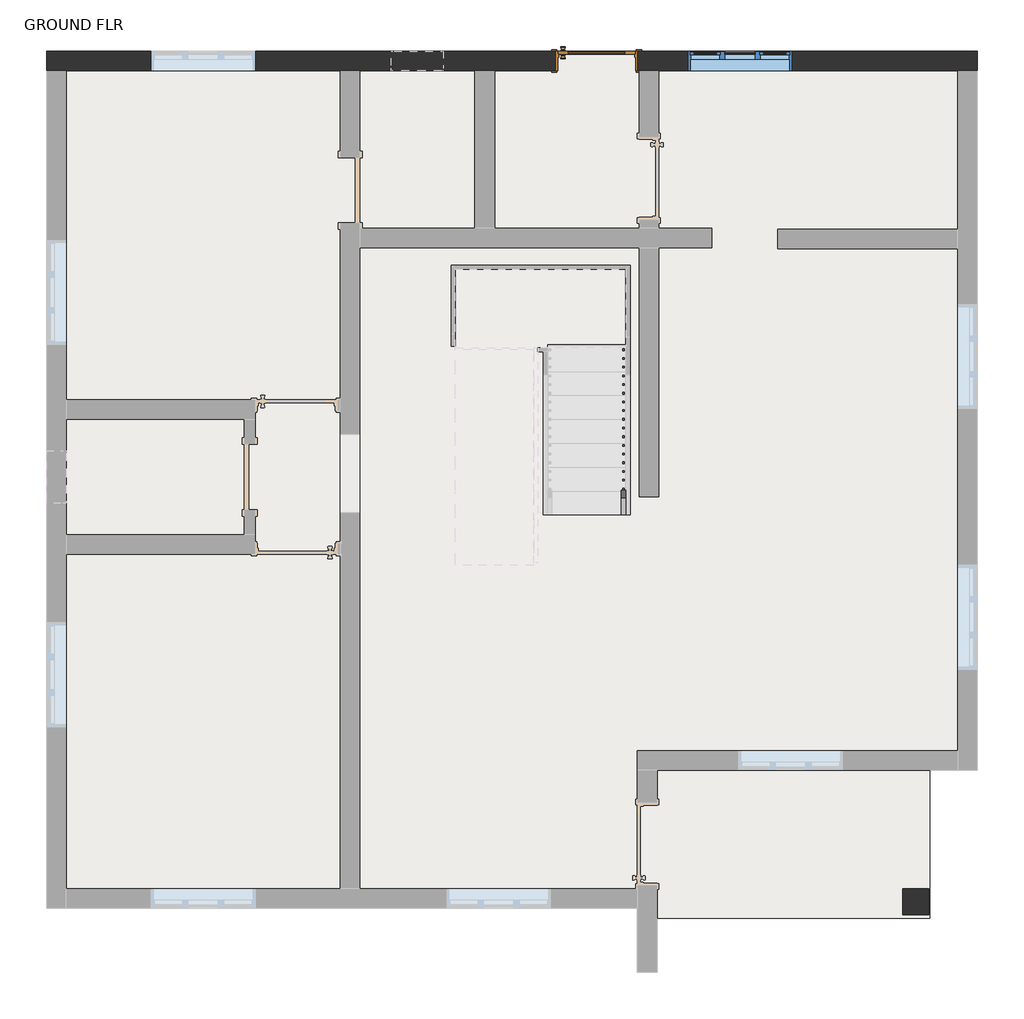
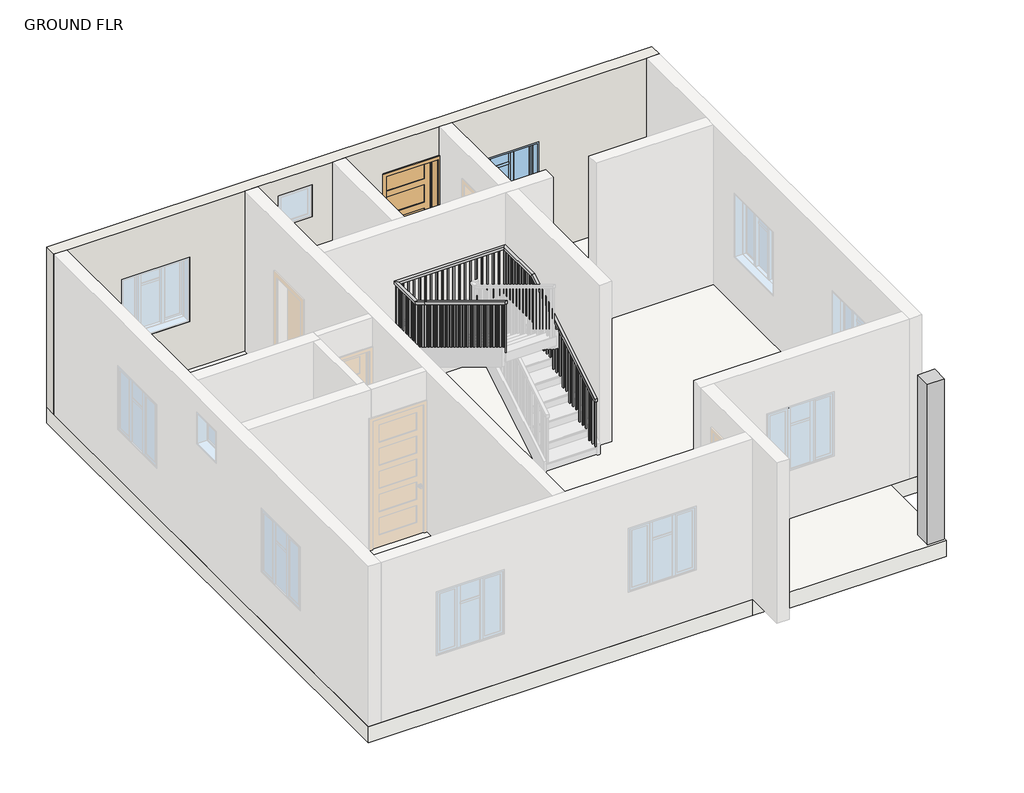
# One storey, part 2 of 3: 1 column, 1 door, 1 railing, 1 slab, 1 wall, 1 window.
"""IFC4 building model written with IfcOpenShell, lengths in millimetres."""

from ifc_helpers import new_model, si_unit, frame, origin, place, context, project, spatial, polyline, outline, extrude, faceted_brep, transform, mapped, element, save
from components import rectangular_column_1_x_1_0efb18cf, door_d793c26e, window_casement_triple_middle_transom_window_4_x_4_1416bf83

model = new_model("IFC4")

# Units and contexts
model_context = context("Model", 3, world=origin())
ifc_project = project(units=[si_unit("LENGTHUNIT", "METRE", prefix="MILLI")], contexts=[model_context])

# Site, building, storey
site = spatial("IfcSite", under=ifc_project)
building = spatial("IfcBuilding", under=site)
storey = spatial("IfcBuildingStorey", under=building, Name="GROUND FLR", Elevation=609.6)

# Column
placement = place(None, origin())
rectangular_column_1_x_1_shape = rectangular_column_1_x_1_0efb18cf(model_context)
element("IfcColumn", 1, ObjectType="Rectangular Column : 1' x 1'", at=placement, inside=storey, context=model_context, shape_type="MappedRepresentation", body=[
    mapped(rectangular_column_1_x_1_shape, transform((-1992.6206632, -7773.7948807, 0.0), x_axis=(1.0, 0.0, 0.0), y_axis=(0.0, 1.0, 0.0), z_axis=(0.0, 0.0, 1.0))),
])

# Door
door_shape = door_d793c26e(model_context)
element("IfcDoor", 2, ObjectType="Door-Interior-Single-5_Panel_Vert-Wood : 36\" x 96\"", at=placement, inside=storey, context=model_context, shape_type="MappedRepresentation", body=[
    mapped(door_shape, transform((-5721.0431792, 2059.1801193, 609.6), x_axis=(1.0, 0.0, 0.0), y_axis=(0.0, 1.0, 0.0), z_axis=(0.0, 0.0, 1.0))),
])

# Railing
element("IfcRailing", 3, ObjectType="Handrail - Rectangular", at=placement, inside=storey, context=model_context, shape_type="SolidModel", body=[
    faceted_brep([(-5431.2481169, -3250.5249317, 1693.3333333), (-5431.2481169, -3250.5249317, 1633.9318731), (-5380.4481169, -3250.5249317, 1633.9318731), (-5380.4481169, -3250.5249317, 1693.3333333), (-5431.2481169, -1294.7249317, 2878.6666667), (-5431.2481169, -1280.5325223, 2827.8666667), (-5380.4481169, -1280.5325223, 2827.8666667), (-5380.4481169, -1294.7249317, 2878.6666667), (-5431.2481169, -431.1249317, 2878.6666667), (-5431.2481169, -431.1249317, 2827.8666667), (-5380.4481169, -380.3249317, 2827.8666667), (-5380.4481169, -380.3249317, 2878.6666667), (-7321.2431792, -431.1249317, 2878.6666667), (-7321.2431792, -431.1249317, 2827.8666667), (-7372.0431792, -380.3249317, 2827.8666667), (-7372.0431792, -380.3249317, 2878.6666667), (-7321.2431792, -1015.3249317, 2878.6666667), (-7321.2431792, -1029.5173411, 2827.8666667), (-7372.0431792, -1029.5173411, 2827.8666667), (-7372.0431792, -1015.3249317, 2878.6666667), (-7321.2431792, -1294.7249317, 3048.0), (-7321.2431792, -1321.0546589, 3004.5559502), (-7372.0431792, -1321.0546589, 3004.5559502), (-7372.0431792, -1294.7249317, 3048.0), (-7321.2431792, -3809.3249317, 4572.0), (-7372.0431792, -3809.3249317, 4572.0), (-7372.0431792, -3809.3249317, 4512.5985397), (-7321.2431792, -3809.3249317, 4512.5985397)], [[[0, 1, 2, 3]], [[1, 0, 4, 5]], [[2, 1, 5, 6]], [[3, 2, 6, 7]], [[0, 3, 7, 4]], [[5, 4, 8, 9]], [[6, 5, 9, 10]], [[7, 6, 10, 11]], [[4, 7, 11, 8]], [[9, 8, 12, 13]], [[10, 9, 13, 14]], [[11, 10, 14, 15]], [[8, 11, 15, 12]], [[13, 12, 16, 17]], [[14, 13, 17, 18]], [[15, 14, 18, 19]], [[12, 15, 19, 16]], [[17, 16, 20, 21]], [[18, 17, 21, 22]], [[19, 18, 22, 23]], [[16, 19, 23, 20]], [[24, 25, 26, 27]], [[21, 20, 24, 27]], [[22, 21, 27, 26]], [[23, 22, 26, 25]], [[20, 23, 25, 24]]]),
    extrude(outline(polyline([(-3742.6499317, 4472.1894488), (-3723.5999317, 4460.6439943), (-3723.5999317, 3488.2666667), (-3742.6499317, 3488.2666667), (-3742.6499317, 4472.1894488)])), frame((-7356.1681792, 0.0, 0.0), z_axis=(1.0, 0.0, 0.0), x_axis=(0.0, 1.0, 0.0)), (0.0, 0.0, 1.0), 19.05),
    extrude(outline(polyline([(-3641.0499317, 4410.6136913), (-3621.9999317, 4399.0682367), (-3621.9999317, 3488.2666667), (-3641.0499317, 3488.2666667), (-3641.0499317, 4410.6136913)])), frame((-7356.1681792, 0.0, 0.0), z_axis=(1.0, 0.0, 0.0), x_axis=(0.0, 1.0, 0.0)), (0.0, 0.0, 1.0), 19.05),
    extrude(outline(polyline([(-3539.4499317, 4349.0379337), (-3520.3999317, 4337.4924791), (-3520.3999317, 3488.2666667), (-3539.4499317, 3488.2666667), (-3539.4499317, 4349.0379337)])), frame((-7356.1681792, 0.0, 0.0), z_axis=(1.0, 0.0, 0.0), x_axis=(0.0, 1.0, 0.0)), (0.0, 0.0, 1.0), 19.05),
    extrude(outline(polyline([(-3437.8499317, 4287.4621761), (-3418.7999317, 4275.9167216), (-3418.7999317, 3318.9333333), (-3437.8499317, 3318.9333333), (-3437.8499317, 4287.4621761)])), frame((-7356.1681792, 0.0, 0.0), z_axis=(1.0, 0.0, 0.0), x_axis=(0.0, 1.0, 0.0)), (0.0, 0.0, 1.0), 19.05),
    extrude(outline(polyline([(-3336.2499317, 4225.8864185), (-3317.1999317, 4214.340964), (-3317.1999317, 3318.9333333), (-3336.2499317, 3318.9333333), (-3336.2499317, 4225.8864185)])), frame((-7356.1681792, 0.0, 0.0), z_axis=(1.0, 0.0, 0.0), x_axis=(0.0, 1.0, 0.0)), (0.0, 0.0, 1.0), 19.05),
    extrude(outline(polyline([(-3234.6499317, 4164.310661), (-3215.5999317, 4152.7652064), (-3215.5999317, 3149.6), (-3234.6499317, 3149.6), (-3234.6499317, 4164.310661)])), frame((-7356.1681792, 0.0, 0.0), z_axis=(1.0, 0.0, 0.0), x_axis=(0.0, 1.0, 0.0)), (0.0, 0.0, 1.0), 19.05),
    extrude(outline(polyline([(-3133.0499317, 4102.7349034), (-3113.9999317, 4091.1894488), (-3113.9999317, 3149.6), (-3133.0499317, 3149.6), (-3133.0499317, 4102.7349034)])), frame((-7356.1681792, 0.0, 0.0), z_axis=(1.0, 0.0, 0.0), x_axis=(0.0, 1.0, 0.0)), (0.0, 0.0, 1.0), 19.05),
    extrude(outline(polyline([(-3031.4499317, 4041.1591458), (-3012.3999317, 4029.6136913), (-3012.3999317, 3149.6), (-3031.4499317, 3149.6), (-3031.4499317, 4041.1591458)])), frame((-7356.1681792, 0.0, 0.0), z_axis=(1.0, 0.0, 0.0), x_axis=(0.0, 1.0, 0.0)), (0.0, 0.0, 1.0), 19.05),
    extrude(outline(polyline([(-2929.8499317, 3979.5833882), (-2910.7999317, 3968.0379337), (-2910.7999317, 2980.2666667), (-2929.8499317, 2980.2666667), (-2929.8499317, 3979.5833882)])), frame((-7356.1681792, 0.0, 0.0), z_axis=(1.0, 0.0, 0.0), x_axis=(0.0, 1.0, 0.0)), (0.0, 0.0, 1.0), 19.05),
    extrude(outline(polyline([(-2828.2499317, 3918.0076307), (-2809.1999317, 3906.4621761), (-2809.1999317, 2980.2666667), (-2828.2499317, 2980.2666667), (-2828.2499317, 3918.0076307)])), frame((-7356.1681792, 0.0, 0.0), z_axis=(1.0, 0.0, 0.0), x_axis=(0.0, 1.0, 0.0)), (0.0, 0.0, 1.0), 19.05),
    extrude(outline(polyline([(-2726.6499317, 3856.4318731), (-2707.5999317, 3844.8864185), (-2707.5999317, 2980.2666667), (-2726.6499317, 2980.2666667), (-2726.6499317, 3856.4318731)])), frame((-7356.1681792, 0.0, 0.0), z_axis=(1.0, 0.0, 0.0), x_axis=(0.0, 1.0, 0.0)), (0.0, 0.0, 1.0), 19.05),
    extrude(outline(polyline([(-2625.0499317, 3794.8561155), (-2605.9999317, 3783.310661), (-2605.9999317, 2810.9333333), (-2625.0499317, 2810.9333333), (-2625.0499317, 3794.8561155)])), frame((-7356.1681792, 0.0, 0.0), z_axis=(1.0, 0.0, 0.0), x_axis=(0.0, 1.0, 0.0)), (0.0, 0.0, 1.0), 19.05),
    extrude(outline(polyline([(-2523.4499317, 3733.2803579), (-2504.3999317, 3721.7349034), (-2504.3999317, 2810.9333333), (-2523.4499317, 2810.9333333), (-2523.4499317, 3733.2803579)])), frame((-7356.1681792, 0.0, 0.0), z_axis=(1.0, 0.0, 0.0), x_axis=(0.0, 1.0, 0.0)), (0.0, 0.0, 1.0), 19.05),
    extrude(outline(polyline([(-2421.8499317, 3671.7046004), (-2402.7999317, 3660.1591458), (-2402.7999317, 2810.9333333), (-2421.8499317, 2810.9333333), (-2421.8499317, 3671.7046004)])), frame((-7356.1681792, 0.0, 0.0), z_axis=(1.0, 0.0, 0.0), x_axis=(0.0, 1.0, 0.0)), (0.0, 0.0, 1.0), 19.05),
    extrude(outline(polyline([(-2320.2499317, 3610.1288428), (-2301.1999317, 3598.5833882), (-2301.1999317, 2641.6), (-2320.2499317, 2641.6), (-2320.2499317, 3610.1288428)])), frame((-7356.1681792, 0.0, 0.0), z_axis=(1.0, 0.0, 0.0), x_axis=(0.0, 1.0, 0.0)), (0.0, 0.0, 1.0), 19.05),
    extrude(outline(polyline([(-2218.6499317, 3548.5530852), (-2199.5999317, 3537.0076307), (-2199.5999317, 2641.6), (-2218.6499317, 2641.6), (-2218.6499317, 3548.5530852)])), frame((-7356.1681792, 0.0, 0.0), z_axis=(1.0, 0.0, 0.0), x_axis=(0.0, 1.0, 0.0)), (0.0, 0.0, 1.0), 19.05),
    extrude(outline(polyline([(-2117.0499317, 3486.9773276), (-2097.9999317, 3475.4318731), (-2097.9999317, 2472.2666667), (-2117.0499317, 2472.2666667), (-2117.0499317, 3486.9773276)])), frame((-7356.1681792, 0.0, 0.0), z_axis=(1.0, 0.0, 0.0), x_axis=(0.0, 1.0, 0.0)), (0.0, 0.0, 1.0), 19.05),
    extrude(outline(polyline([(-2015.4499317, 3425.40157), (-1996.3999317, 3413.8561155), (-1996.3999317, 2472.2666667), (-2015.4499317, 2472.2666667), (-2015.4499317, 3425.40157)])), frame((-7356.1681792, 0.0, 0.0), z_axis=(1.0, 0.0, 0.0), x_axis=(0.0, 1.0, 0.0)), (0.0, 0.0, 1.0), 19.05),
    extrude(outline(polyline([(-1913.8499317, 3363.8258125), (-1894.7999317, 3352.2803579), (-1894.7999317, 2472.2666667), (-1913.8499317, 2472.2666667), (-1913.8499317, 3363.8258125)])), frame((-7356.1681792, 0.0, 0.0), z_axis=(1.0, 0.0, 0.0), x_axis=(0.0, 1.0, 0.0)), (0.0, 0.0, 1.0), 19.05),
    extrude(outline(polyline([(-1812.2499317, 3302.2500549), (-1793.1999317, 3290.7046004), (-1793.1999317, 2302.9333333), (-1812.2499317, 2302.9333333), (-1812.2499317, 3302.2500549)])), frame((-7356.1681792, 0.0, 0.0), z_axis=(1.0, 0.0, 0.0), x_axis=(0.0, 1.0, 0.0)), (0.0, 0.0, 1.0), 19.05),
    extrude(outline(polyline([(-1710.6499317, 3240.6742973), (-1691.5999317, 3229.1288428), (-1691.5999317, 2302.9333333), (-1710.6499317, 2302.9333333), (-1710.6499317, 3240.6742973)])), frame((-7356.1681792, 0.0, 0.0), z_axis=(1.0, 0.0, 0.0), x_axis=(0.0, 1.0, 0.0)), (0.0, 0.0, 1.0), 19.05),
    extrude(outline(polyline([(-1609.0499317, 3179.0985397), (-1589.9999317, 3167.5530852), (-1589.9999317, 2302.9333333), (-1609.0499317, 2302.9333333), (-1609.0499317, 3179.0985397)])), frame((-7356.1681792, 0.0, 0.0), z_axis=(1.0, 0.0, 0.0), x_axis=(0.0, 1.0, 0.0)), (0.0, 0.0, 1.0), 19.05),
    extrude(outline(polyline([(-1507.4499317, 3117.5227822), (-1488.3999317, 3105.9773276), (-1488.3999317, 2133.6), (-1507.4499317, 2133.6), (-1507.4499317, 3117.5227822)])), frame((-7356.1681792, 0.0, 0.0), z_axis=(1.0, 0.0, 0.0), x_axis=(0.0, 1.0, 0.0)), (0.0, 0.0, 1.0), 19.05),
    extrude(outline(polyline([(-1405.8499317, 3055.9470246), (-1386.7999317, 3044.40157), (-1386.7999317, 2133.6), (-1405.8499317, 2133.6), (-1405.8499317, 3055.9470246)])), frame((-7356.1681792, 0.0, 0.0), z_axis=(1.0, 0.0, 0.0), x_axis=(0.0, 1.0, 0.0)), (0.0, 0.0, 1.0), 19.05),
    extrude(outline(polyline([(-1228.0499317, 2948.1894488), (-1208.9999317, 2936.6439943), (-1208.9999317, 1964.2666667), (-1228.0499317, 1964.2666667), (-1228.0499317, 2948.1894488)])), frame((-7356.1681792, 0.0, 0.0), z_axis=(1.0, 0.0, 0.0), x_axis=(0.0, 1.0, 0.0)), (0.0, 0.0, 1.0), 19.05),
    extrude(outline(polyline([(-1126.4499317, 2886.6136913), (-1107.3999317, 2875.0682367), (-1107.3999317, 1964.2666667), (-1126.4499317, 1964.2666667), (-1126.4499317, 2886.6136913)])), frame((-7356.1681792, 0.0, 0.0), z_axis=(1.0, 0.0, 0.0), x_axis=(0.0, 1.0, 0.0)), (0.0, 0.0, 1.0), 19.05),
    extrude(outline(polyline([(-7356.1681792, -1005.7999317), (-7337.1181792, -1005.7999317), (-7337.1181792, -1024.8499317), (-7356.1681792, -1024.8499317), (-7356.1681792, -1005.7999317)])), frame((0.0, 0.0, 1964.2666667), z_axis=(0.0, 0.0, 1.0), x_axis=(1.0, 0.0, 0.0)), (0.0, 0.0, 1.0), 863.6),
    extrude(outline(polyline([(-7356.1681792, -904.1999317), (-7337.1181792, -904.1999317), (-7337.1181792, -923.2499317), (-7356.1681792, -923.2499317), (-7356.1681792, -904.1999317)])), frame((0.0, 0.0, 1964.2666667), z_axis=(0.0, 0.0, 1.0), x_axis=(1.0, 0.0, 0.0)), (0.0, 0.0, 1.0), 863.6),
    extrude(outline(polyline([(-7356.1681792, -802.5999317), (-7337.1181792, -802.5999317), (-7337.1181792, -821.6499317), (-7356.1681792, -821.6499317), (-7356.1681792, -802.5999317)])), frame((0.0, 0.0, 1964.2666667), z_axis=(0.0, 0.0, 1.0), x_axis=(1.0, 0.0, 0.0)), (0.0, 0.0, 1.0), 863.6),
    extrude(outline(polyline([(-7356.1681792, -700.9999317), (-7337.1181792, -700.9999317), (-7337.1181792, -720.0499317), (-7356.1681792, -720.0499317), (-7356.1681792, -700.9999317)])), frame((0.0, 0.0, 1964.2666667), z_axis=(0.0, 0.0, 1.0), x_axis=(1.0, 0.0, 0.0)), (0.0, 0.0, 1.0), 863.6),
    extrude(outline(polyline([(-7356.1681792, -599.3999317), (-7337.1181792, -599.3999317), (-7337.1181792, -618.4499317), (-7356.1681792, -618.4499317), (-7356.1681792, -599.3999317)])), frame((0.0, 0.0, 1964.2666667), z_axis=(0.0, 0.0, 1.0), x_axis=(1.0, 0.0, 0.0)), (0.0, 0.0, 1.0), 863.6),
    extrude(outline(polyline([(-7356.1681792, -497.7999317), (-7337.1181792, -497.7999317), (-7337.1181792, -516.8499317), (-7356.1681792, -516.8499317), (-7356.1681792, -497.7999317)])), frame((0.0, 0.0, 1964.2666667), z_axis=(0.0, 0.0, 1.0), x_axis=(1.0, 0.0, 0.0)), (0.0, 0.0, 1.0), 863.6),
    extrude(outline(polyline([(-7326.7231169, -396.1999317), (-7326.7231169, -415.2499317), (-7345.7731169, -415.2499317), (-7345.7731169, -396.1999317), (-7326.7231169, -396.1999317)])), frame((0.0, 0.0, 1964.2666667), z_axis=(0.0, 0.0, 1.0), x_axis=(1.0, 0.0, 0.0)), (0.0, 0.0, 1.0), 863.6),
    extrude(outline(polyline([(-7225.1231169, -396.1999317), (-7225.1231169, -415.2499317), (-7244.1731169, -415.2499317), (-7244.1731169, -396.1999317), (-7225.1231169, -396.1999317)])), frame((0.0, 0.0, 1964.2666667), z_axis=(0.0, 0.0, 1.0), x_axis=(1.0, 0.0, 0.0)), (0.0, 0.0, 1.0), 863.6),
    extrude(outline(polyline([(-7123.5231169, -396.1999317), (-7123.5231169, -415.2499317), (-7142.5731169, -415.2499317), (-7142.5731169, -396.1999317), (-7123.5231169, -396.1999317)])), frame((0.0, 0.0, 1964.2666667), z_axis=(0.0, 0.0, 1.0), x_axis=(1.0, 0.0, 0.0)), (0.0, 0.0, 1.0), 863.6),
    extrude(outline(polyline([(-7021.9231169, -396.1999317), (-7021.9231169, -415.2499317), (-7040.9731169, -415.2499317), (-7040.9731169, -396.1999317), (-7021.9231169, -396.1999317)])), frame((0.0, 0.0, 1964.2666667), z_axis=(0.0, 0.0, 1.0), x_axis=(1.0, 0.0, 0.0)), (0.0, 0.0, 1.0), 863.6),
    extrude(outline(polyline([(-6920.3231169, -396.1999317), (-6920.3231169, -415.2499317), (-6939.3731169, -415.2499317), (-6939.3731169, -396.1999317), (-6920.3231169, -396.1999317)])), frame((0.0, 0.0, 1964.2666667), z_axis=(0.0, 0.0, 1.0), x_axis=(1.0, 0.0, 0.0)), (0.0, 0.0, 1.0), 863.6),
    extrude(outline(polyline([(-6818.7231169, -396.1999317), (-6818.7231169, -415.2499317), (-6837.7731169, -415.2499317), (-6837.7731169, -396.1999317), (-6818.7231169, -396.1999317)])), frame((0.0, 0.0, 1964.2666667), z_axis=(0.0, 0.0, 1.0), x_axis=(1.0, 0.0, 0.0)), (0.0, 0.0, 1.0), 863.6),
    extrude(outline(polyline([(-6717.1231169, -396.1999317), (-6717.1231169, -415.2499317), (-6736.1731169, -415.2499317), (-6736.1731169, -396.1999317), (-6717.1231169, -396.1999317)])), frame((0.0, 0.0, 1964.2666667), z_axis=(0.0, 0.0, 1.0), x_axis=(1.0, 0.0, 0.0)), (0.0, 0.0, 1.0), 863.6),
    extrude(outline(polyline([(-6615.5231169, -396.1999317), (-6615.5231169, -415.2499317), (-6634.5731169, -415.2499317), (-6634.5731169, -396.1999317), (-6615.5231169, -396.1999317)])), frame((0.0, 0.0, 1964.2666667), z_axis=(0.0, 0.0, 1.0), x_axis=(1.0, 0.0, 0.0)), (0.0, 0.0, 1.0), 863.6),
    extrude(outline(polyline([(-6513.9231169, -396.1999317), (-6513.9231169, -415.2499317), (-6532.9731169, -415.2499317), (-6532.9731169, -396.1999317), (-6513.9231169, -396.1999317)])), frame((0.0, 0.0, 1964.2666667), z_axis=(0.0, 0.0, 1.0), x_axis=(1.0, 0.0, 0.0)), (0.0, 0.0, 1.0), 863.6),
    extrude(outline(polyline([(-6412.3231169, -396.1999317), (-6412.3231169, -415.2499317), (-6431.3731169, -415.2499317), (-6431.3731169, -396.1999317), (-6412.3231169, -396.1999317)])), frame((0.0, 0.0, 1964.2666667), z_axis=(0.0, 0.0, 1.0), x_axis=(1.0, 0.0, 0.0)), (0.0, 0.0, 1.0), 863.6),
    extrude(outline(polyline([(-6310.7231169, -396.1999317), (-6310.7231169, -415.2499317), (-6329.7731169, -415.2499317), (-6329.7731169, -396.1999317), (-6310.7231169, -396.1999317)])), frame((0.0, 0.0, 1964.2666667), z_axis=(0.0, 0.0, 1.0), x_axis=(1.0, 0.0, 0.0)), (0.0, 0.0, 1.0), 863.6),
    extrude(outline(polyline([(-6209.1231169, -396.1999317), (-6209.1231169, -415.2499317), (-6228.1731169, -415.2499317), (-6228.1731169, -396.1999317), (-6209.1231169, -396.1999317)])), frame((0.0, 0.0, 1964.2666667), z_axis=(0.0, 0.0, 1.0), x_axis=(1.0, 0.0, 0.0)), (0.0, 0.0, 1.0), 863.6),
    extrude(outline(polyline([(-6107.5231169, -396.1999317), (-6107.5231169, -415.2499317), (-6126.5731169, -415.2499317), (-6126.5731169, -396.1999317), (-6107.5231169, -396.1999317)])), frame((0.0, 0.0, 1964.2666667), z_axis=(0.0, 0.0, 1.0), x_axis=(1.0, 0.0, 0.0)), (0.0, 0.0, 1.0), 863.6),
    extrude(outline(polyline([(-6005.9231169, -396.1999317), (-6005.9231169, -415.2499317), (-6024.9731169, -415.2499317), (-6024.9731169, -396.1999317), (-6005.9231169, -396.1999317)])), frame((0.0, 0.0, 1964.2666667), z_axis=(0.0, 0.0, 1.0), x_axis=(1.0, 0.0, 0.0)), (0.0, 0.0, 1.0), 863.6),
    extrude(outline(polyline([(-5904.3231169, -396.1999317), (-5904.3231169, -415.2499317), (-5923.3731169, -415.2499317), (-5923.3731169, -396.1999317), (-5904.3231169, -396.1999317)])), frame((0.0, 0.0, 1964.2666667), z_axis=(0.0, 0.0, 1.0), x_axis=(1.0, 0.0, 0.0)), (0.0, 0.0, 1.0), 863.6),
    extrude(outline(polyline([(-5802.7231169, -396.1999317), (-5802.7231169, -415.2499317), (-5821.7731169, -415.2499317), (-5821.7731169, -396.1999317), (-5802.7231169, -396.1999317)])), frame((0.0, 0.0, 1964.2666667), z_axis=(0.0, 0.0, 1.0), x_axis=(1.0, 0.0, 0.0)), (0.0, 0.0, 1.0), 863.6),
    extrude(outline(polyline([(-5701.1231169, -396.1999317), (-5701.1231169, -415.2499317), (-5720.1731169, -415.2499317), (-5720.1731169, -396.1999317), (-5701.1231169, -396.1999317)])), frame((0.0, 0.0, 1964.2666667), z_axis=(0.0, 0.0, 1.0), x_axis=(1.0, 0.0, 0.0)), (0.0, 0.0, 1.0), 863.6),
    extrude(outline(polyline([(-5599.5231169, -396.1999317), (-5599.5231169, -415.2499317), (-5618.5731169, -415.2499317), (-5618.5731169, -396.1999317), (-5599.5231169, -396.1999317)])), frame((0.0, 0.0, 1964.2666667), z_axis=(0.0, 0.0, 1.0), x_axis=(1.0, 0.0, 0.0)), (0.0, 0.0, 1.0), 863.6),
    extrude(outline(polyline([(-5497.9231169, -396.1999317), (-5497.9231169, -415.2499317), (-5516.9731169, -415.2499317), (-5516.9731169, -396.1999317), (-5497.9231169, -396.1999317)])), frame((0.0, 0.0, 1964.2666667), z_axis=(0.0, 0.0, 1.0), x_axis=(1.0, 0.0, 0.0)), (0.0, 0.0, 1.0), 863.6),
    extrude(outline(polyline([(-5396.3231169, -491.4499317), (-5415.3731169, -491.4499317), (-5415.3731169, -472.3999317), (-5396.3231169, -472.3999317), (-5396.3231169, -491.4499317)])), frame((0.0, 0.0, 1964.2666667), z_axis=(0.0, 0.0, 1.0), x_axis=(1.0, 0.0, 0.0)), (0.0, 0.0, 1.0), 863.6),
    extrude(outline(polyline([(-5396.3231169, -593.0499317), (-5415.3731169, -593.0499317), (-5415.3731169, -573.9999317), (-5396.3231169, -573.9999317), (-5396.3231169, -593.0499317)])), frame((0.0, 0.0, 1964.2666667), z_axis=(0.0, 0.0, 1.0), x_axis=(1.0, 0.0, 0.0)), (0.0, 0.0, 1.0), 863.6),
    extrude(outline(polyline([(-5396.3231169, -694.6499317), (-5415.3731169, -694.6499317), (-5415.3731169, -675.5999317), (-5396.3231169, -675.5999317), (-5396.3231169, -694.6499317)])), frame((0.0, 0.0, 1964.2666667), z_axis=(0.0, 0.0, 1.0), x_axis=(1.0, 0.0, 0.0)), (0.0, 0.0, 1.0), 863.6),
    extrude(outline(polyline([(-5396.3231169, -796.2499317), (-5415.3731169, -796.2499317), (-5415.3731169, -777.1999317), (-5396.3231169, -777.1999317), (-5396.3231169, -796.2499317)])), frame((0.0, 0.0, 1964.2666667), z_axis=(0.0, 0.0, 1.0), x_axis=(1.0, 0.0, 0.0)), (0.0, 0.0, 1.0), 863.6),
    extrude(outline(polyline([(-5396.3231169, -897.8499317), (-5415.3731169, -897.8499317), (-5415.3731169, -878.7999317), (-5396.3231169, -878.7999317), (-5396.3231169, -897.8499317)])), frame((0.0, 0.0, 1964.2666667), z_axis=(0.0, 0.0, 1.0), x_axis=(1.0, 0.0, 0.0)), (0.0, 0.0, 1.0), 863.6),
    extrude(outline(polyline([(-5396.3231169, -999.4499317), (-5415.3731169, -999.4499317), (-5415.3731169, -980.3999317), (-5396.3231169, -980.3999317), (-5396.3231169, -999.4499317)])), frame((0.0, 0.0, 1964.2666667), z_axis=(0.0, 0.0, 1.0), x_axis=(1.0, 0.0, 0.0)), (0.0, 0.0, 1.0), 863.6),
    extrude(outline(polyline([(-5396.3231169, -1101.0499317), (-5415.3731169, -1101.0499317), (-5415.3731169, -1081.9999317), (-5396.3231169, -1081.9999317), (-5396.3231169, -1101.0499317)])), frame((0.0, 0.0, 1964.2666667), z_axis=(0.0, 0.0, 1.0), x_axis=(1.0, 0.0, 0.0)), (0.0, 0.0, 1.0), 863.6),
    extrude(outline(polyline([(-5396.3231169, -1202.6499317), (-5415.3731169, -1202.6499317), (-5415.3731169, -1183.5999317), (-5396.3231169, -1183.5999317), (-5396.3231169, -1202.6499317)])), frame((0.0, 0.0, 1964.2666667), z_axis=(0.0, 0.0, 1.0), x_axis=(1.0, 0.0, 0.0)), (0.0, 0.0, 1.0), 863.6),
    extrude(outline(polyline([(-1329.6499317, 2798.0985397), (-1310.5999317, 2809.6439943), (-1310.5999317, 1794.9333333), (-1329.6499317, 1794.9333333), (-1329.6499317, 2798.0985397)])), frame((-5415.3731169, 0.0, 0.0), z_axis=(1.0, 0.0, 0.0), x_axis=(0.0, 1.0, 0.0)), (0.0, 0.0, 1.0), 19.05),
    extrude(outline(polyline([(-1431.2499317, 2736.5227822), (-1412.1999317, 2748.0682367), (-1412.1999317, 1794.9333333), (-1431.2499317, 1794.9333333), (-1431.2499317, 2736.5227822)])), frame((-5415.3731169, 0.0, 0.0), z_axis=(1.0, 0.0, 0.0), x_axis=(0.0, 1.0, 0.0)), (0.0, 0.0, 1.0), 19.05),
    extrude(outline(polyline([(-1532.8499317, 2674.9470246), (-1513.7999317, 2686.4924791), (-1513.7999317, 1794.9333333), (-1532.8499317, 1794.9333333), (-1532.8499317, 2674.9470246)])), frame((-5415.3731169, 0.0, 0.0), z_axis=(1.0, 0.0, 0.0), x_axis=(0.0, 1.0, 0.0)), (0.0, 0.0, 1.0), 19.05),
    extrude(outline(polyline([(-1634.4499317, 2613.371267), (-1615.3999317, 2624.9167216), (-1615.3999317, 1625.6), (-1634.4499317, 1625.6), (-1634.4499317, 2613.371267)])), frame((-5415.3731169, 0.0, 0.0), z_axis=(1.0, 0.0, 0.0), x_axis=(0.0, 1.0, 0.0)), (0.0, 0.0, 1.0), 19.05),
    extrude(outline(polyline([(-1736.0499317, 2551.7955094), (-1716.9999317, 2563.340964), (-1716.9999317, 1625.6), (-1736.0499317, 1625.6), (-1736.0499317, 2551.7955094)])), frame((-5415.3731169, 0.0, 0.0), z_axis=(1.0, 0.0, 0.0), x_axis=(0.0, 1.0, 0.0)), (0.0, 0.0, 1.0), 19.05),
    extrude(outline(polyline([(-1837.6499317, 2490.2197519), (-1818.5999317, 2501.7652064), (-1818.5999317, 1625.6), (-1837.6499317, 1625.6), (-1837.6499317, 2490.2197519)])), frame((-5415.3731169, 0.0, 0.0), z_axis=(1.0, 0.0, 0.0), x_axis=(0.0, 1.0, 0.0)), (0.0, 0.0, 1.0), 19.05),
    extrude(outline(polyline([(-1939.2499317, 2428.6439943), (-1920.1999317, 2440.1894488), (-1920.1999317, 1456.2666667), (-1939.2499317, 1456.2666667), (-1939.2499317, 2428.6439943)])), frame((-5415.3731169, 0.0, 0.0), z_axis=(1.0, 0.0, 0.0), x_axis=(0.0, 1.0, 0.0)), (0.0, 0.0, 1.0), 19.05),
    extrude(outline(polyline([(-2040.8499317, 2367.0682367), (-2021.7999317, 2378.6136913), (-2021.7999317, 1456.2666667), (-2040.8499317, 1456.2666667), (-2040.8499317, 2367.0682367)])), frame((-5415.3731169, 0.0, 0.0), z_axis=(1.0, 0.0, 0.0), x_axis=(0.0, 1.0, 0.0)), (0.0, 0.0, 1.0), 19.05),
    extrude(outline(polyline([(-2142.4499317, 2305.4924791), (-2123.3999317, 2317.0379337), (-2123.3999317, 1456.2666667), (-2142.4499317, 1456.2666667), (-2142.4499317, 2305.4924791)])), frame((-5415.3731169, 0.0, 0.0), z_axis=(1.0, 0.0, 0.0), x_axis=(0.0, 1.0, 0.0)), (0.0, 0.0, 1.0), 19.05),
    extrude(outline(polyline([(-2244.0499317, 2243.9167216), (-2224.9999317, 2255.4621761), (-2224.9999317, 1286.9333333), (-2244.0499317, 1286.9333333), (-2244.0499317, 2243.9167216)])), frame((-5415.3731169, 0.0, 0.0), z_axis=(1.0, 0.0, 0.0), x_axis=(0.0, 1.0, 0.0)), (0.0, 0.0, 1.0), 19.05),
    extrude(outline(polyline([(-2345.6499317, 2182.340964), (-2326.5999317, 2193.8864185), (-2326.5999317, 1286.9333333), (-2345.6499317, 1286.9333333), (-2345.6499317, 2182.340964)])), frame((-5415.3731169, 0.0, 0.0), z_axis=(1.0, 0.0, 0.0), x_axis=(0.0, 1.0, 0.0)), (0.0, 0.0, 1.0), 19.05),
    extrude(outline(polyline([(-2447.2499317, 2120.7652064), (-2428.1999317, 2132.310661), (-2428.1999317, 1117.6), (-2447.2499317, 1117.6), (-2447.2499317, 2120.7652064)])), frame((-5415.3731169, 0.0, 0.0), z_axis=(1.0, 0.0, 0.0), x_axis=(0.0, 1.0, 0.0)), (0.0, 0.0, 1.0), 19.05),
    extrude(outline(polyline([(-2548.8499317, 2059.1894488), (-2529.7999317, 2070.7349034), (-2529.7999317, 1117.6), (-2548.8499317, 1117.6), (-2548.8499317, 2059.1894488)])), frame((-5415.3731169, 0.0, 0.0), z_axis=(1.0, 0.0, 0.0), x_axis=(0.0, 1.0, 0.0)), (0.0, 0.0, 1.0), 19.05),
    extrude(outline(polyline([(-2650.4499317, 1997.6136913), (-2631.3999317, 2009.1591458), (-2631.3999317, 1117.6), (-2650.4499317, 1117.6), (-2650.4499317, 1997.6136913)])), frame((-5415.3731169, 0.0, 0.0), z_axis=(1.0, 0.0, 0.0), x_axis=(0.0, 1.0, 0.0)), (0.0, 0.0, 1.0), 19.05),
    extrude(outline(polyline([(-2752.0499317, 1936.0379337), (-2732.9999317, 1947.5833882), (-2732.9999317, 948.2666667), (-2752.0499317, 948.2666667), (-2752.0499317, 1936.0379337)])), frame((-5415.3731169, 0.0, 0.0), z_axis=(1.0, 0.0, 0.0), x_axis=(0.0, 1.0, 0.0)), (0.0, 0.0, 1.0), 19.05),
    extrude(outline(polyline([(-2853.6499317, 1874.4621761), (-2834.5999317, 1886.0076307), (-2834.5999317, 948.2666667), (-2853.6499317, 948.2666667), (-2853.6499317, 1874.4621761)])), frame((-5415.3731169, 0.0, 0.0), z_axis=(1.0, 0.0, 0.0), x_axis=(0.0, 1.0, 0.0)), (0.0, 0.0, 1.0), 19.05),
    extrude(outline(polyline([(-2955.2499317, 1812.8864185), (-2936.1999317, 1824.4318731), (-2936.1999317, 948.2666667), (-2955.2499317, 948.2666667), (-2955.2499317, 1812.8864185)])), frame((-5415.3731169, 0.0, 0.0), z_axis=(1.0, 0.0, 0.0), x_axis=(0.0, 1.0, 0.0)), (0.0, 0.0, 1.0), 19.05),
    extrude(outline(polyline([(-3056.8499317, 1751.310661), (-3037.7999317, 1762.8561155), (-3037.7999317, 778.9333333), (-3056.8499317, 778.9333333), (-3056.8499317, 1751.310661)])), frame((-5415.3731169, 0.0, 0.0), z_axis=(1.0, 0.0, 0.0), x_axis=(0.0, 1.0, 0.0)), (0.0, 0.0, 1.0), 19.05),
    extrude(outline(polyline([(-3158.4499317, 1689.7349034), (-3139.3999317, 1701.2803579), (-3139.3999317, 778.9333333), (-3158.4499317, 778.9333333), (-3158.4499317, 1689.7349034)])), frame((-5415.3731169, 0.0, 0.0), z_axis=(1.0, 0.0, 0.0), x_axis=(0.0, 1.0, 0.0)), (0.0, 0.0, 1.0), 19.05),
    extrude(outline(polyline([(-1304.2499317, 2994.371267), (-1285.1999317, 2982.8258125), (-1285.1999317, 1964.2666667), (-1304.2499317, 1964.2666667), (-1304.2499317, 2994.371267)])), frame((-7356.1681792, 0.0, 0.0), z_axis=(1.0, 0.0, 0.0), x_axis=(0.0, 1.0, 0.0)), (0.0, 0.0, 1.0), 19.05),
    extrude(outline(polyline([(-7337.1181792, -396.1999317), (-7337.1181792, -415.2499317), (-7356.1681792, -415.2499317), (-7356.1681792, -396.1999317), (-7337.1181792, -396.1999317)])), frame((0.0, 0.0, 1964.2666667), z_axis=(0.0, 0.0, 1.0), x_axis=(1.0, 0.0, 0.0)), (0.0, 0.0, 1.0), 863.6),
    extrude(outline(polyline([(-5396.3231169, -415.2499317), (-5415.3731169, -415.2499317), (-5415.3731169, -396.1999317), (-5396.3231169, -396.1999317), (-5396.3231169, -415.2499317)])), frame((0.0, 0.0, 1964.2666667), z_axis=(0.0, 0.0, 1.0), x_axis=(1.0, 0.0, 0.0)), (0.0, 0.0, 1.0), 863.6),
    extrude(outline(polyline([(-1304.2499317, 2813.4924791), (-1285.1999317, 2825.0379337), (-1285.1999317, 1964.2666667), (-1304.2499317, 1964.2666667), (-1304.2499317, 2813.4924791)])), frame((-5415.3731169, 0.0, 0.0), z_axis=(1.0, 0.0, 0.0), x_axis=(0.0, 1.0, 0.0)), (0.0, 0.0, 1.0), 19.05),
    extrude(outline(polyline([(-3809.3249317, 4512.5985397), (-3790.2749317, 4501.0530852), (-3790.2749317, 3488.2666667), (-3809.3249317, 3488.2666667), (-3809.3249317, 4512.5985397)])), frame((-7356.1681792, 0.0, 0.0), z_axis=(1.0, 0.0, 0.0), x_axis=(0.0, 1.0, 0.0)), (0.0, 0.0, 1.0), 19.05),
    extrude(outline(polyline([(-3250.5249317, 1633.9318731), (-3231.4749317, 1645.4773276), (-3231.4749317, 778.9333333), (-3250.5249317, 778.9333333), (-3250.5249317, 1633.9318731)])), frame((-5415.3731169, 0.0, 0.0), z_axis=(1.0, 0.0, 0.0), x_axis=(0.0, 1.0, 0.0)), (0.0, 0.0, 1.0), 19.05),
])

# Slab
element("IfcSlab", 4, ObjectType="Generic - 12\"", at=placement, inside=storey, context=model_context, shape_type="SweptSolid", body=[
    extrude(outline(polyline([(-12152.6206632, -7849.9948807), (-12152.6206632, 2170.3051193), (-1268.7206632, 2170.3051193), (-1268.7206632, -6237.0948807), (-1827.5206632, -6237.0948807), (-1827.5206632, -7964.2948807), (-5015.2206632, -7964.2948807), (-5015.2206632, -7849.9948807), (-5243.8206632, -7849.9948807), (-12152.6206632, -7849.9948807)])), frame((0.0, 0.0, 304.8), z_axis=(0.0, 0.0, 1.0), x_axis=(1.0, 0.0, 0.0)), (0.0, 0.0, 1.0), 304.8),
])

# Wall
element("IfcWall", 5, ObjectType="WALL 9\"", at=placement, inside=storey, context=model_context, shape_type="Brep", body=[
    faceted_brep([(-1268.7206632, 1941.7051193, 3657.6), (-1497.3206632, 1941.7051193, 3657.6), (-4997.1431792, 1941.7051193, 3657.6), (-5225.7431792, 1941.7051193, 3657.6), (-6914.8431792, 1941.7051193, 3657.6), (-7143.4431792, 1941.7051193, 3657.6), (-8489.6431792, 1941.7051193, 3657.6), (-8718.2431792, 1941.7051193, 3657.6), (-11924.0206632, 1941.7051193, 3657.6), (-12152.6206632, 1941.7051193, 3657.6), (-12152.6206632, 1941.7051193, 609.6), (-11924.0206632, 1941.7051193, 609.6), (-8718.2431792, 1941.7051193, 609.6), (-8489.6431792, 1941.7051193, 609.6), (-7143.4431792, 1941.7051193, 609.6), (-6914.8431792, 1941.7051193, 609.6), (-6203.6431792, 1941.7051193, 609.6), (-6203.6431792, 1941.7051193, 3073.4), (-5238.4431792, 1941.7051193, 3073.4), (-5238.4431792, 1941.7051193, 609.6), (-5225.7431792, 1941.7051193, 609.6), (-4997.1431792, 1941.7051193, 609.6), (-1497.3206632, 1941.7051193, 609.6), (-1268.7206632, 1941.7051193, 609.6), (-9711.5319212, 1941.7051193, 2743.2), (-9711.5319212, 1941.7051193, 1524.0), (-10930.7319212, 1941.7051193, 1524.0), (-10930.7319212, 1941.7051193, 2743.2), (-3435.0431792, 1941.7051193, 2743.2), (-3435.0431792, 1941.7051193, 1524.0), (-4654.2431792, 1941.7051193, 1524.0), (-4654.2431792, 1941.7051193, 2743.2), (-8121.3431792, 1941.7051193, 3352.8), (-7511.7431792, 1941.7051193, 3352.8), (-7511.7431792, 1941.7051193, 2743.2), (-8121.3431792, 1941.7051193, 2743.2), (-12152.6206632, 2170.3051193, 3657.6), (-1268.7206632, 2170.3051193, 3657.6), (-1268.7206632, 2170.3051193, 609.6), (-5238.4431792, 2170.3051193, 609.6), (-5238.4431792, 2170.3051193, 3073.4), (-6203.6431792, 2170.3051193, 3073.4), (-6203.6431792, 2170.3051193, 609.6), (-12152.6206632, 2170.3051193, 609.6), (-9711.5319212, 2170.3051193, 2743.2), (-10930.7319212, 2170.3051193, 2743.2), (-10930.7319212, 2170.3051193, 1524.0), (-9711.5319212, 2170.3051193, 1524.0), (-3435.0431792, 2170.3051193, 2743.2), (-4654.2431792, 2170.3051193, 2743.2), (-4654.2431792, 2170.3051193, 1524.0), (-3435.0431792, 2170.3051193, 1524.0), (-8121.3431792, 2170.3051193, 3352.8), (-8121.3431792, 2170.3051193, 2743.2), (-7511.7431792, 2170.3051193, 2743.2), (-7511.7431792, 2170.3051193, 3352.8)], [[[0, 1, 2, 3, 4, 5, 6, 7, 8, 9, 10, 11, 12, 13, 14, 15, 16, 17, 18, 19, 20, 21, 22, 23], [24, 25, 26, 27], [28, 29, 30, 31], [32, 33, 34, 35]], [[36, 37, 38, 39, 40, 41, 42, 43], [44, 45, 46, 47], [48, 49, 50, 51], [52, 53, 54, 55]], [[10, 43, 42, 16, 15, 14, 13, 12, 11]], [[38, 23, 22, 21, 20, 19, 39]], [[9, 8, 7, 6, 5, 4, 3, 2, 1, 0, 37, 36]], [[10, 9, 36, 43]], [[0, 23, 38, 37]], [[18, 40, 39, 19]], [[40, 18, 17, 41]], [[41, 17, 16, 42]], [[25, 24, 44, 47]], [[26, 25, 47, 46]], [[27, 26, 46, 45]], [[24, 27, 45, 44]], [[29, 28, 48, 51]], [[30, 29, 51, 50]], [[31, 30, 50, 49]], [[28, 31, 49, 48]], [[53, 52, 32, 35]], [[54, 53, 35, 34]], [[55, 54, 34, 33]], [[52, 55, 33, 32]]]),
])

# Window
window_casement_triple_middle_transom_window_4_x_4_shape = window_casement_triple_middle_transom_window_4_x_4_1416bf83(model_context)
element("IfcWindow", 6, ObjectType="Window-Casement-Triple-Middle-Transom : WINDOW 4' X 4'", at=placement, inside=storey, context=model_context, shape_type="MappedRepresentation", body=[
    mapped(window_casement_triple_middle_transom_window_4_x_4_shape, transform((-4044.6431792, 2056.0051193, 609.6), x_axis=(1.0, 0.0, 0.0), y_axis=(0.0, 1.0, 0.0), z_axis=(0.0, 0.0, 1.0))),
])

save(model, "model.ifc")

# Revit data of these elements
# Type "Rectangular Column : 1' x 1'"
#   Assembly Code = "B1010200"
#   Depth = 1' - 0"
#   Offset Base = 0' - 0"
#   Offset Top = 0' - 0"
#   Width = 1' - 0"
#   Material = SOFT COOL PAINT
# Type "Door-Interior-Single-5_Panel_Vert-Wood : 36\" x 96\""
#   Type Mark = "8"
#   Assembly Code = "C1020300"
#   Analytic Construction = "Wooden"
#   Top Rail = 0' - 4 11/16"
#   Thickness = 0' - 1 3/8"
#   Thermal Resistance (R) = 2.5876 (h·ft²·°F)/BTU
#   Swing Angle [instance default] = 90.00°
#   Stiles = 0' - 4 3/4"
#   Rough Width = 3' - 2"
#   Rough Height = 8' - 1"
#   Intermediate Rail = 0' - 4 1/2"
#   Height = 8' - 0"
#   Width = 3' - 0"
#   Heat Transfer Coefficient (U) = 0.3865 BTU/(h·ft²·°F)
#   Bottom Rail = 0' - 9 1/8"
#   Trim Material = Cherry
#   Panel Material = Cherry
#   Frame Material = Cherry
#   Door Handle Material = Aluminum
#   Visual Light Transmittance = 0
#   Solar Heat Gain Coefficient = 0
#   Wall Closure = (empty or 0)
#   Function = (empty or 0)
# Type "Handrail - Rectangular"
#   Assembly Code = "C2010400"
#   built-in parameter 1008612 = 0.0416667 (stored number, unit not read)
#   built-in parameter 1008611 = 0.0416667 (stored number, unit not read)
#   built-in parameter 1008609 = 0.333333 (stored number, unit not read)
#   built-in parameter 1008604 = 0.166667 (stored number, unit not read)
#   built-in parameter 1008603 = 0.166667 (stored number, unit not read)
#   Railing Height = 3' - 0"
#   built-in parameter 1008630 = 2
#   built-in parameter 1008610 = 2
#   built-in parameter 1008618 = Baluster - Square : 3/4"
# Type "Generic - 12\""
#   Assembly Code = "B1010"
#   Function = 0
#   Layers, outside or top first: 1' - 0" no material (function 1)
# Type "WALL 9\""
#   Assembly Code = "B2010"
#   Layers, outside or top first: 0' - 9" "SOFT COOL PAINT" (function 1)
# Type "Window-Casement-Triple-Middle-Transom : WINDOW 4' X 4'"
#   Type Mark = "21"
#   Fire Rating = "0.5h"
#   Assembly Code = "B2020100"
#   Analytic Construction = "Double glazing - domestic"
#   Window Width = 1' - 4"
#   Window Inset [instance default] = 0' - 0 5/8"
#   Wall Thickness [instance default] = 0' - 6"
#   Visual Light Transmittance = 0.81
#   Transom Height Ratio = 0.3
#   Thermal Resistance (R) = 1.8146 (h·ft²·°F)/BTU
#   Solar Heat Gain Coefficient = 0.76
#   Rough Width = 4' - 0 1/2"
#   Rough Height = 4' - 0 1/2"
#   Heat Transfer Coefficient (U) = 0.5511 BTU/(h·ft²·°F)
#   Height = 4' - 0"
#   Transom Height = 1' - 2.4"
#   Frame Gap 3 [instance default] = 0' - 1 83/128"
#   Frame Gap 2 [instance default] = 0' - 0 5/8"
#   Frame Gap 1 = 0' - 1 51/128"
#   Default Sill Height = 3' - 0"
#   Width = 4' - 0"
#   Frame Material = WOOD MATERIAL
#   Glass Panel Material = GLASS MATERIAL
#   Wall Closure = (empty or 0)
# Element 1 (IfcColumn, "Rectangular Column : 1' x 1'")
#   Phase Created = New Construction
#   Materials on its faces: "SOFT COOL PAINT"
# Element 2 (IfcDoor, "Door-Interior-Single-5_Panel_Vert-Wood : 36\" x 96\"")
#   Swing Angle = 90.00°
#   Phase Created = New Construction
#   Materials on its faces: "Cherry", "Aluminum"
# Element 3 (IfcRailing, "Handrail - Rectangular")
#   Phase Created = New Construction
# Element 4 (IfcSlab, "Generic - 12\"")
#   built-in parameter 1001955 = -1.5708 (stored number, unit not read)
#   Height Offset From Level = 0' - 0"
#   Phase Created = New Construction
#   Materials on its faces: "Default Floor"
# Element 5 (IfcWall, "WALL 9\"")
#   Top Offset = 0' - 0"
#   Base Offset = 0' - 0"
#   wall height = 10' - 0"
#   Phase Created = New Construction
#   Base Constraint = GROUND FLR
#   Top Constraint = FIRST FLR
#   Materials on its faces: "SOFT COOL PAINT"
# Element 6 (IfcWindow, "Window-Casement-Triple-Middle-Transom : WINDOW 4' X 4'")
#   Mark = "9"
#   Window Inset = 0' - 0 5/8"
#   Frame Gap 3 = 0' - 1 83/128"
#   Frame Gap 2 = 0' - 0 5/8"
#   Phase Created = New Construction
#   Materials on its faces: "WOOD MATERIAL", "GLASS MATERIAL"
# Materials
#   "SOFT COOL PAINT": class "Generic", colour RGB 120 120 120, transparency 0, Cost = 0
#   "Cherry": class "Wood", colour RGB 226 177 128, transparency 0, Description = "Prunus Serotina", Cost = 0
#   "Aluminum": class "Metal", colour RGB 247 247 247, transparency 0, Description = "Aluminum 6061", Cost = 0
#   "WOOD MATERIAL": class "Generic", colour RGB 120 120 120, transparency 0, Cost = 0
#   "GLASS MATERIAL": class "Generic", colour RGB 120 120 120, transparency 0, Cost = 0
#   "Default Floor": colour RGB 128 128 128, transparency 0, Cost = 0
